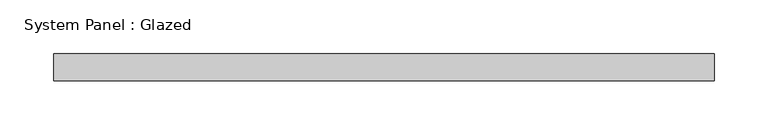
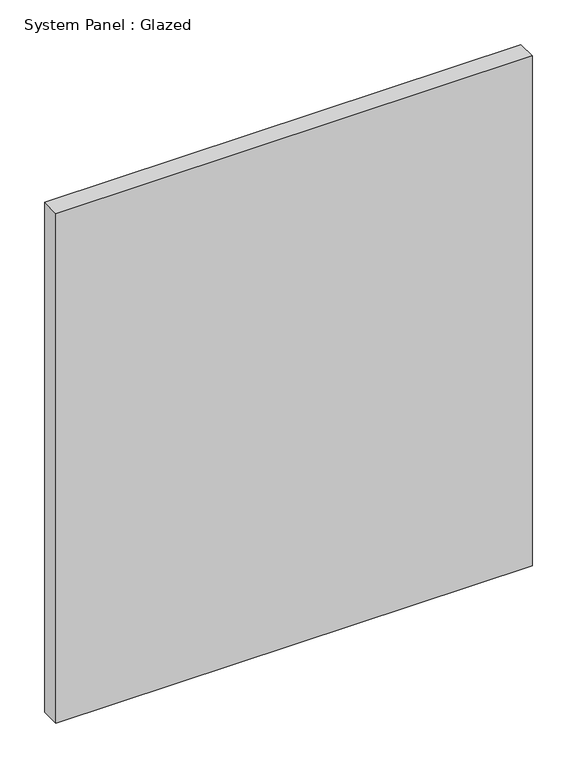
"""IFC4 building model written with IfcOpenShell, lengths in millimetres: plate geometry, System Panel : Glazed."""

from ifc_helpers import new_model, si_unit, origin, origin_with_axes, place, context, project, spatial, polyline, outline, extrude, source, transform, mapped, element, save


def system_panel_glazed_4a2f6317(model_context):
    return source(origin(), model_context, "Body", "SweptSolid", [
        extrude(outline(polyline([(307.975, 19.05), (-307.975, 19.05), (-307.975, 44.45), (307.975, 44.45), (307.975, 19.05)])), origin_with_axes(), (0.0, 0.0, 1.0), 697.350254),
    ])


if __name__ == "__main__":
    model = new_model("IFC4")
    model_context = context("Model", 3, world=origin())
    ifc_project = project(units=[si_unit("LENGTHUNIT", "METRE", prefix="MILLI")], contexts=[model_context])
    site = spatial("IfcSite", under=ifc_project)
    building = spatial("IfcBuilding", under=site)
    placement = place(None, origin())
    system_panel_glazed_shape = system_panel_glazed_4a2f6317(model_context)
    element("IfcPlate", 1, ObjectType="System Panel : Glazed", at=placement, inside=building, context=model_context, shape_type="MappedRepresentation", body=[
        mapped(system_panel_glazed_shape, transform((0.0, 0.0, 0.0), x_axis=(1.0, 0.0, 0.0), y_axis=(0.0, 1.0, 0.0), z_axis=(0.0, 0.0, 1.0))),
    ])
    save(model, "model.ifc")

# Revit data of these elements
# Type "System Panel : Glazed"
#   Construction Type Id = "GSP4R"
#   Analytic Construction = "1/8 in Pilkington single glazing"
#   Visual Light Transmittance = 0.9
#   Solar Heat Gain Coefficient = 0.86
#   Heat Transfer Coefficient (U) = 1.18115 BTU/(h·ft²·°F)
#   Define Thermal Properties by = 1
# Element 1 (IfcPlate, "System Panel : Glazed")
#   Materials on its faces: "Glass"
# Materials
#   "Glass": class "Glass", colour RGB 0 128 192, transparency 0.75, Description = "Soda Lime Glass", Cost = 0
